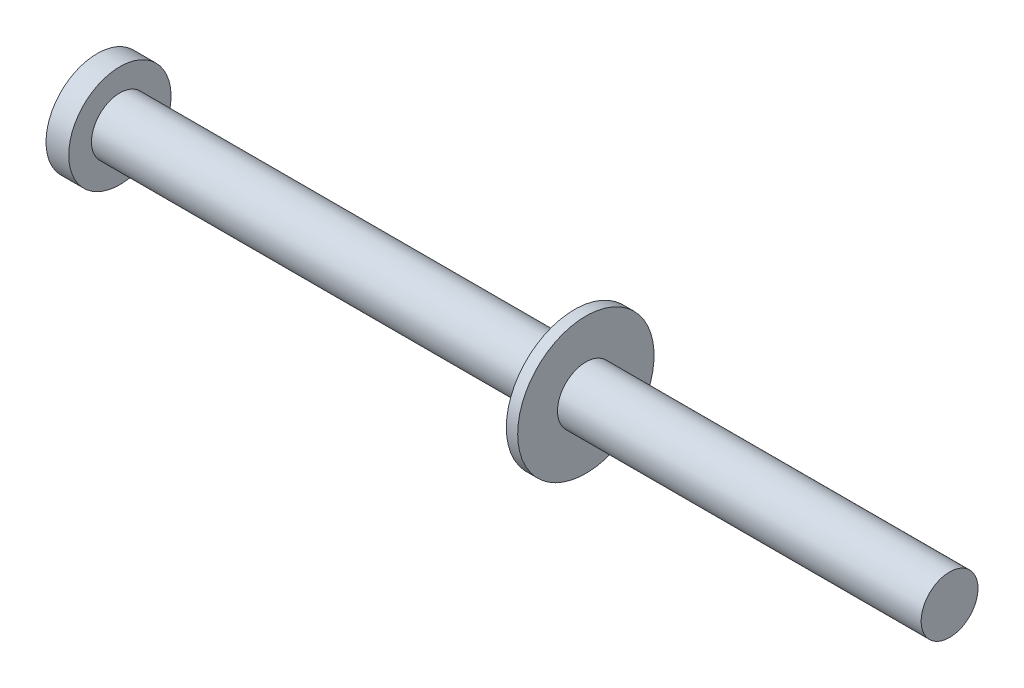
from build123d import *

# Parameters (mm, degrees)
SHAFT_SECTION_A_PROFILE_10_R = 5
SHAFT_SECTION_A_10X64_DEPTH  = 64
COLLAR_PROFILE_24_R          = 12
COLLAR_24X2_DEPTH            = 2
SHAFT_START                  = 80
SHAFT_SECTION_B_PROFILE_10_R = 5
SHAFT_SECTION_B_10X80_DEPTH  = 80
HEAD_PROFILE_18_R            = 9
HEAD_18X4_DEPTH              = 4


with BuildPart() as part:
    # Shaft Section A Profile Ø10 → Shaft Section A Ø10x64 (new body)
    with BuildSketch(Plane(origin=(0, 0, 0), x_dir=(0, 0, -1), z_dir=(1, 0, 0))):
        Circle(SHAFT_SECTION_A_PROFILE_10_R)
    extrude(amount=SHAFT_SECTION_A_10X64_DEPTH)

    # Collar Profile Ø24 → Collar Ø24x2 (add)
    with BuildSketch(Plane.ZY):
        Circle(COLLAR_PROFILE_24_R)
    extrude(amount=COLLAR_24X2_DEPTH)

    # Shaft Section B Profile Ø10 → Shaft Section B Ø10x80 (add)
    with BuildSketch(Plane.ZY.offset(2).offset(SHAFT_START)):
        with Locations(Location((0, 0, 0), (0, 0, 180))):
            Circle(SHAFT_SECTION_B_PROFILE_10_R)
    extrude(amount=-SHAFT_SECTION_B_10X80_DEPTH)

    # Head Profile Ø18 → Head Ø18x4 (add)
    with BuildSketch(Plane.ZY.offset(82)):
        Circle(HEAD_PROFILE_18_R)
    extrude(amount=HEAD_18X4_DEPTH)


solid = part.part
